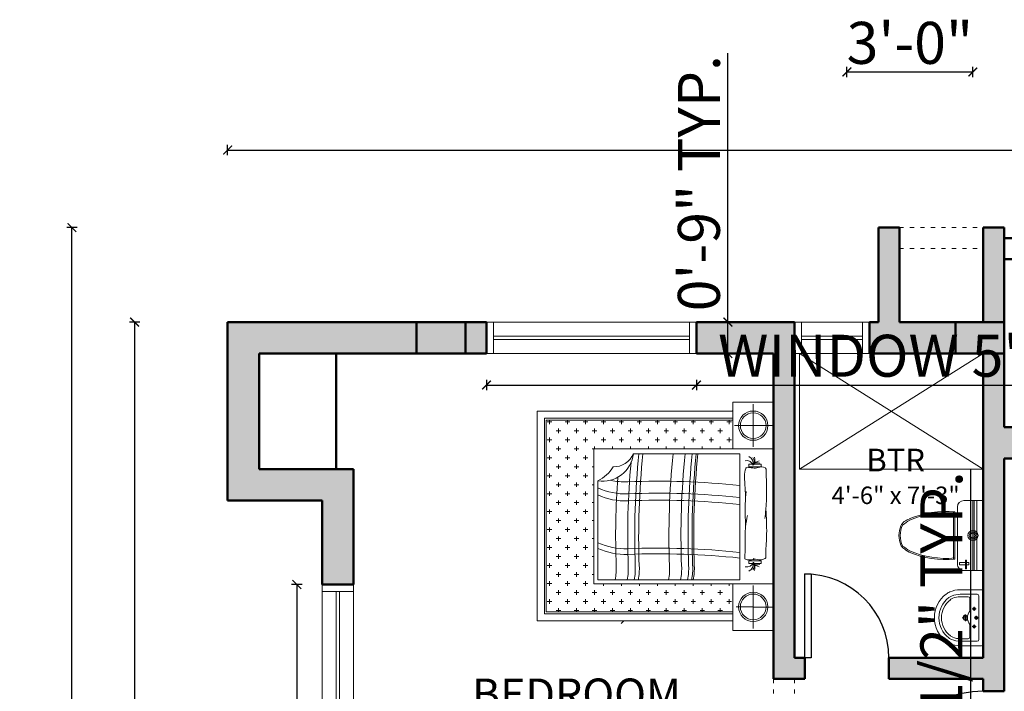
# Model space of a CAD drawing. Units: inches. Extents: x 375 to 1122, y 27 to 1069.
# Tile 77 of 155: x 385 to 667, y 877 to 1069. Entities that reach past the tile are written whole.
import ezdxf

# ---------------------------------------------------------------- set-up
doc = ezdxf.new("R2010")
doc.units = ezdxf.units.IN
doc.linetypes.add('ACAD_ISO03W100', pattern=[30, 12, -18])
for name, color, linetype, lineweight in [('A-ANNO-DIMS', 2, 'Continuous', 18), ('A-AREA-IDEN', 7, 'Continuous', 18), ('A-COLS-PATT', 10, 'Continuous', 13), ('A-FLOR-FIXT', 55, 'Continuous', 18), ('A-WALL-OVHD', 77, 'ACAD_ISO03W100', 18), ('A-WALL-PATT', 252, 'Continuous', 13), ('Columns', 10, 'Continuous', 50), ('Doors', 150, 'Continuous', 25), ('Furniture', 30, 'Continuous', 18), ('Shower Areas', 53, 'Continuous', 18), ('Walls', 250, 'Continuous', 50), ('Windows', 122, 'Continuous', 18)]:
    doc.layers.add(name, color=color, linetype=linetype, lineweight=lineweight)
doc.styles.get("Standard").update_dxf_attribs({"font": 'arial.ttf'})
doc.dimstyles.new('ISO-25', dxfattribs={"dimtxt": 12, "dimasz": 2.5, "dimexe": 1.5, "dimexo": 1.5, "dimtad": 1, "dimdec": 1, "dimlunit": 3, "dimtxsty": 'Standard', "dimblk": 'ARCHTICK', "dimcen": 2.5, "dimadec": 0, "dimazin": 0, "dimtfac": 1, "dimtdec": 1, "dimtmove": 0, "dimatfit": 3, "dimfxl": 1.5, "dimfxlon": 1, "dimarcsym": 0})

# ---------------------------------------------------------------- blocks, each defined once
blk = doc.blocks.new('*U7')
for p, q in [((0, 0), (0, -4)), ((24, 0), (24, -4))]:
    blk.add_line(p, q)
blk.add_lwpolyline([(0, 0), (0, 24), (1.75, 24), (1.75, 0)], close=True)
blk.add_arc((0, 0), 24, 0, 90)
blk = doc.blocks.new('*U10')
for p, q in [((-30, 0), (-30, 4)), ((0, 0), (0, 4))]:
    blk.add_line(p, q)
blk.add_lwpolyline([(0, 0), (0, -30), (-1.75, -30), (-1.75, 0)], close=True)
blk.add_arc((0, 0), 30, 180, 270)
blk = doc.blocks.new('A$C52B64FF5')
for p, q in [((0.522, 2.628), (0, 2.628)), ((0, 2.628), (0, 2.178)), ((0.262, 2.403), (0.262, 2.616)), ((0.522, 2.178), (0.522, 2.628)), ((2.022, 2.628), (0.522, 2.628)), ((0.522, 2.628), (0.522, 0.628)), ((2.543, 2.628), (2.022, 2.628)), ((2.022, 0.628), (2.022, 2.628)), ((2.022, 2.628), (2.022, 2.178)), ((2.282, 2.403), (2.282, 2.616)), ((2.543, 2.178), (2.543, 2.628)), ((0.721, 2.493), (0.692, 2.493)), ((0.692, 2.493), (0.692, 2.353)), ((0.721, 2.353), (0.721, 2.493)), ((1.767, 2.353), (1.767, 2.493)), ((1.767, 2.493), (1.796, 2.493)), ((1.796, 2.493), (1.796, 2.353)), ((0.263, 2.403), (0.023, 2.403)), ((0.023, 2.403), (0.5, 2.403)), ((0.263, 2.195), (0.263, 2.403)), ((0.692, 2.353), (0.721, 2.353)), ((1.796, 2.353), (1.767, 2.353)), ((2.52, 2.403), (2.043, 2.403)), ((2.28, 2.213), (2.28, 2.403)), ((2.28, 2.403), (2.52, 2.403)), ((0.575, 1.068), (0.575, 2.254)), ((0.575, 2.254), (1.978, 2.254)), ((1.978, 2.254), (1.978, 0.675)), ((0, 2.178), (0.522, 2.178)), ((0.093, 2.178), (0.101, 2.17)), ((0.101, 0), (0.101, 2.178)), ((0.181, 0.08), (0.181, 2.178)), ((0.201, 0.1), (0.201, 2.178)), ((0.201, 2.136), (0.245, 2.136)), ((0.22, 2.111), (0.22, 2.161)), ((0.395, 2.136), (0.445, 2.136)), ((0.42, 2.111), (0.42, 2.161)), ((2.543, 2.178), (2.022, 2.178)), ((2.022, 2.178), (2.543, 2.178)), ((2.022, 2.136), (2.045, 2.136)), ((2.195, 2.136), (2.245, 2.136)), ((2.22, 2.111), (2.22, 2.161)), ((2.337, 2.178), (2.337, 0.1)), ((2.357, 2.178), (2.357, 0.08)), ((2.437, 2.178), (2.437, 0)), ((0.295, 2.036), (0.345, 2.036)), ((0.32, 2.011), (0.32, 2.061)), ((0.495, 2.036), (0.522, 2.036)), ((0.52, 2.011), (0.52, 2.061)), ((2.095, 2.036), (2.145, 2.036)), ((2.12, 2.011), (2.12, 2.061)), ((2.295, 2.036), (2.337, 2.036)), ((2.32, 2.011), (2.32, 2.061)), ((0.201, 1.936), (0.245, 1.936)), ((0.22, 1.911), (0.22, 1.961)), ((0.395, 1.936), (0.445, 1.936)), ((0.42, 1.911), (0.42, 1.961)), ((2.022, 1.936), (2.045, 1.936)), ((2.195, 1.936), (2.245, 1.936)), ((2.22, 1.911), (2.22, 1.961)), ((0.22, 1.711), (0.22, 1.761)), ((0.295, 1.836), (0.345, 1.836)), ((0.32, 1.811), (0.32, 1.861)), ((0.42, 1.711), (0.42, 1.761)), ((0.495, 1.836), (0.522, 1.836)), ((0.52, 1.811), (0.52, 1.861)), ((2.095, 1.836), (2.145, 1.836)), ((2.12, 1.811), (2.12, 1.861)), ((2.22, 1.711), (2.22, 1.761)), ((2.295, 1.836), (2.337, 1.836)), ((2.32, 1.811), (2.32, 1.861)), ((0.201, 1.736), (0.245, 1.736)), ((0.32, 1.611), (0.32, 1.661)), ((0.395, 1.736), (0.445, 1.736)), ((0.52, 1.611), (0.52, 1.661)), ((2.022, 1.736), (2.045, 1.736)), ((2.12, 1.611), (2.12, 1.661)), ((2.195, 1.736), (2.245, 1.736)), ((2.32, 1.611), (2.32, 1.661)), ((0.201, 1.536), (0.245, 1.536)), ((0.22, 1.511), (0.22, 1.561)), ((0.295, 1.636), (0.345, 1.636)), ((0.395, 1.536), (0.445, 1.536)), ((0.42, 1.511), (0.42, 1.561)), ((0.495, 1.636), (0.522, 1.636)), ((2.022, 1.536), (2.045, 1.536)), ((2.095, 1.636), (2.145, 1.636)), ((2.195, 1.536), (2.245, 1.536)), ((2.22, 1.511), (2.22, 1.561)), ((2.295, 1.636), (2.337, 1.636)), ((0.295, 1.436), (0.345, 1.436)), ((0.32, 1.411), (0.32, 1.461)), ((0.495, 1.436), (0.522, 1.436)), ((0.52, 1.411), (0.52, 1.461)), ((2.095, 1.436), (2.145, 1.436)), ((2.12, 1.411), (2.12, 1.461)), ((2.295, 1.436), (2.337, 1.436)), ((2.32, 1.411), (2.32, 1.461)), ((0.201, 1.336), (0.245, 1.336)), ((0.22, 1.311), (0.22, 1.361)), ((0.395, 1.336), (0.445, 1.336)), ((0.42, 1.311), (0.42, 1.361)), ((2.022, 1.336), (2.045, 1.336)), ((2.195, 1.336), (2.245, 1.336)), ((2.22, 1.311), (2.22, 1.361)), ((0.295, 1.236), (0.345, 1.236)), ((0.32, 1.211), (0.32, 1.261)), ((0.495, 1.236), (0.522, 1.236)), ((0.52, 1.211), (0.52, 1.261)), ((2.095, 1.236), (2.145, 1.236)), ((2.12, 1.211), (2.12, 1.261)), ((2.295, 1.236), (2.337, 1.236)), ((2.32, 1.211), (2.32, 1.261)), ((0.201, 1.136), (0.245, 1.136)), ((0.22, 1.111), (0.22, 1.161)), ((0.395, 1.136), (0.445, 1.136)), ((0.42, 1.111), (0.42, 1.161)), ((2.022, 1.136), (2.045, 1.136)), ((2.195, 1.136), (2.245, 1.136)), ((2.22, 1.111), (2.22, 1.161)), ((0.295, 1.036), (0.345, 1.036)), ((0.32, 1.011), (0.32, 1.061)), ((0.495, 1.036), (0.522, 1.036)), ((0.52, 1.011), (0.52, 1.061)), ((2.095, 1.036), (2.145, 1.036)), ((2.12, 1.011), (2.12, 1.061)), ((2.295, 1.036), (2.337, 1.036)), ((2.32, 1.011), (2.32, 1.061)), ((0.201, 0.936), (0.245, 0.936)), ((0.22, 0.911), (0.22, 0.961)), ((0.395, 0.936), (0.445, 0.936)), ((0.42, 0.911), (0.42, 0.961)), ((2.022, 0.936), (2.045, 0.936)), ((2.195, 0.936), (2.245, 0.936)), ((2.22, 0.911), (2.22, 0.961)), ((2.437, 0.962), (2.464, 0.935)), ((0.295, 0.836), (0.345, 0.836)), ((0.32, 0.811), (0.32, 0.861)), ((0.495, 0.836), (0.522, 0.836)), ((0.52, 0.811), (0.52, 0.861)), ((2.095, 0.836), (2.145, 0.836)), ((2.12, 0.811), (2.12, 0.861)), ((2.295, 0.836), (2.337, 0.836)), ((2.32, 0.811), (2.32, 0.861)), ((0.201, 0.736), (0.245, 0.736)), ((0.22, 0.711), (0.22, 0.761)), ((0.32, 0.611), (0.32, 0.661)), ((0.395, 0.736), (0.445, 0.736)), ((0.42, 0.711), (0.42, 0.761)), ((0.52, 0.611), (0.52, 0.661)), ((1.978, 0.675), (0.876, 0.675)), ((2.022, 0.736), (2.045, 0.736)), ((2.12, 0.611), (2.12, 0.661)), ((2.195, 0.736), (2.245, 0.736)), ((2.22, 0.711), (2.22, 0.761)), ((2.32, 0.611), (2.32, 0.661)), ((0.22, 0.511), (0.22, 0.561)), ((0.295, 0.636), (0.345, 0.636)), ((0.42, 0.511), (0.42, 0.561)), ((0.495, 0.636), (0.522, 0.636)), ((0.522, 0.628), (2.022, 0.628)), ((0.62, 0.511), (0.62, 0.561)), ((0.72, 0.611), (0.72, 0.628)), ((0.82, 0.511), (0.82, 0.561)), ((0.92, 0.611), (0.92, 0.628)), ((1.02, 0.511), (1.02, 0.561)), ((1.12, 0.611), (1.12, 0.628)), ((1.22, 0.511), (1.22, 0.561)), ((1.32, 0.611), (1.32, 0.628)), ((1.42, 0.511), (1.42, 0.561)), ((1.52, 0.611), (1.52, 0.628)), ((1.62, 0.511), (1.62, 0.561)), ((1.72, 0.611), (1.72, 0.628)), ((1.82, 0.511), (1.82, 0.561)), ((1.92, 0.611), (1.92, 0.628)), ((2.02, 0.511), (2.02, 0.561)), ((2.095, 0.636), (2.145, 0.636)), ((2.22, 0.511), (2.22, 0.561)), ((2.295, 0.636), (2.337, 0.636)), ((0.201, 0.536), (0.245, 0.536)), ((0.32, 0.411), (0.32, 0.461)), ((0.395, 0.536), (0.445, 0.536)), ((0.52, 0.411), (0.52, 0.461)), ((0.595, 0.536), (0.645, 0.536)), ((0.72, 0.411), (0.72, 0.461)), ((0.795, 0.536), (0.845, 0.536)), ((0.92, 0.411), (0.92, 0.461)), ((0.995, 0.536), (1.045, 0.536)), ((1.12, 0.411), (1.12, 0.461)), ((1.195, 0.536), (1.245, 0.536)), ((1.32, 0.411), (1.32, 0.461)), ((1.395, 0.536), (1.445, 0.536)), ((1.52, 0.411), (1.52, 0.461)), ((1.595, 0.536), (1.645, 0.536)), ((1.72, 0.411), (1.72, 0.461)), ((1.795, 0.536), (1.845, 0.536)), ((1.92, 0.411), (1.92, 0.461)), ((1.995, 0.536), (2.045, 0.536)), ((2.12, 0.411), (2.12, 0.461)), ((2.195, 0.536), (2.245, 0.536)), ((2.32, 0.411), (2.32, 0.461)), ((0.201, 0.336), (0.245, 0.336)), ((0.22, 0.311), (0.22, 0.361)), ((0.295, 0.436), (0.345, 0.436)), ((0.395, 0.336), (0.445, 0.336)), ((0.42, 0.311), (0.42, 0.361)), ((0.495, 0.436), (0.545, 0.436)), ((0.595, 0.336), (0.645, 0.336)), ((0.62, 0.311), (0.62, 0.361)), ((0.695, 0.436), (0.745, 0.436)), ((0.795, 0.336), (0.845, 0.336)), ((0.82, 0.311), (0.82, 0.361)), ((0.895, 0.436), (0.945, 0.436)), ((0.995, 0.336), (1.045, 0.336)), ((1.02, 0.311), (1.02, 0.361)), ((1.095, 0.436), (1.145, 0.436)), ((1.195, 0.336), (1.245, 0.336)), ((1.22, 0.311), (1.22, 0.361)), ((1.295, 0.436), (1.345, 0.436)), ((1.395, 0.336), (1.445, 0.336)), ((1.42, 0.311), (1.42, 0.361)), ((1.495, 0.436), (1.545, 0.436)), ((1.595, 0.336), (1.645, 0.336)), ((1.62, 0.311), (1.62, 0.361)), ((1.695, 0.436), (1.745, 0.436)), ((1.795, 0.336), (1.845, 0.336)), ((1.82, 0.311), (1.82, 0.361)), ((1.895, 0.436), (1.945, 0.436)), ((1.995, 0.336), (2.045, 0.336)), ((2.02, 0.311), (2.02, 0.361)), ((2.095, 0.436), (2.145, 0.436)), ((2.195, 0.336), (2.245, 0.336)), ((2.22, 0.311), (2.22, 0.361)), ((2.295, 0.436), (2.337, 0.436)), ((0.295, 0.236), (0.345, 0.236)), ((0.32, 0.211), (0.32, 0.261)), ((0.495, 0.236), (0.545, 0.236)), ((0.52, 0.211), (0.52, 0.261)), ((0.695, 0.236), (0.745, 0.236)), ((0.72, 0.211), (0.72, 0.261)), ((0.895, 0.236), (0.945, 0.236)), ((0.92, 0.211), (0.92, 0.261)), ((1.095, 0.236), (1.145, 0.236)), ((1.12, 0.211), (1.12, 0.261)), ((1.295, 0.236), (1.345, 0.236)), ((1.32, 0.211), (1.32, 0.261)), ((1.495, 0.236), (1.545, 0.236)), ((1.52, 0.211), (1.52, 0.261)), ((1.695, 0.236), (1.745, 0.236)), ((1.72, 0.211), (1.72, 0.261)), ((1.895, 0.236), (1.945, 0.236)), ((1.92, 0.211), (1.92, 0.261)), ((2.095, 0.236), (2.145, 0.236)), ((2.12, 0.211), (2.12, 0.261)), ((2.295, 0.236), (2.337, 0.236)), ((2.32, 0.211), (2.32, 0.261)), ((0.201, 0.136), (0.245, 0.136)), ((0.22, 0.111), (0.22, 0.161)), ((0.395, 0.136), (0.445, 0.136)), ((0.42, 0.111), (0.42, 0.161)), ((0.595, 0.136), (0.645, 0.136)), ((0.62, 0.111), (0.62, 0.161)), ((0.795, 0.136), (0.845, 0.136)), ((0.82, 0.111), (0.82, 0.161)), ((0.995, 0.136), (1.045, 0.136)), ((1.02, 0.111), (1.02, 0.161)), ((1.195, 0.136), (1.245, 0.136)), ((1.22, 0.111), (1.22, 0.161)), ((1.395, 0.136), (1.445, 0.136)), ((1.42, 0.111), (1.42, 0.161)), ((1.595, 0.136), (1.645, 0.136)), ((1.62, 0.111), (1.62, 0.161)), ((1.795, 0.136), (1.845, 0.136)), ((1.82, 0.111), (1.82, 0.161)), ((1.995, 0.136), (2.045, 0.136)), ((2.02, 0.111), (2.02, 0.161)), ((2.195, 0.136), (2.245, 0.136)), ((2.22, 0.111), (2.22, 0.161)), ((2.437, 0), (0.101, 0)), ((2.357, 0.08), (0.181, 0.08)), ((2.337, 0.1), (0.201, 0.1))]:
    blk.add_line(p, q)
for centre, radius in [((0.263, 2.403), 0.163), ((0.263, 2.403), 0.143), ((2.28, 2.403), 0.163), ((2.28, 2.403), 0.143)]:
    blk.add_circle(centre, radius)
for centre, radius, start, end in [((0.644, 2.315), 0.107, 59.2174, 107.2401), ((0.665, 2.321), 0.0913, 67.8398, 120.4859), ((0.752, 2.492), 0.101, 192.774, 239.2386), ((0.757, 2.452), 0.0808, 161.4559, 221.5545), ((1.736, 2.492), 0.101, 300.7614, 347.226), ((1.844, 2.315), 0.107, 72.7599, 120.7826), ((1.823, 2.321), 0.0913, 59.5141, 112.1602), ((1.732, 2.452), 0.0808, 318.4455, 18.5441), ((0.689, 2.306), 0.098, 80.9486, 149.4879), ((0.729, 2.33), 0.0776, 109.2642, 192.2669), ((1.759, 2.33), 0.0776, 347.7331, 73.8836), ((1.799, 2.306), 0.098, 30.5121, 99.0514), ((9.729, 1.341), 8.848, 174.0754, 182.1662), ((9.863, 1.341), 8.848, 174.0754, 182.1662), ((9.941, 1.341), 8.848, 174.0754, 182.1662), ((10.474, 1.341), 8.848, 174.0754, 182.1662), ((10.537, 1.341), 8.848, 174.0754, 182.1662), ((1.488, 10.589), 8.848, 264.0754, 272.1662), ((1.488, 10.57), 8.848, 264.0754, 272.1662), ((1.488, 10.526), 8.848, 264.0754, 272.1662), ((1.488, 10.447), 8.848, 264.0754, 272.1662), ((1.85, 1.028), 0.72, 79.7409, 92.1662), ((1.85, 1.01), 0.72, 79.7409, 92.1662), ((1.85, 0.965), 0.72, 79.7409, 92.1662), ((1.85, 0.887), 0.72, 79.7409, 92.1662), ((1.488, 10.313), 8.848, 264.0754, 272.1662), ((1.85, 0.753), 0.72, 79.7409, 92.1662), ((1.488, 9.976), 8.848, 264.0754, 272.1662), ((1.488, 9.932), 8.848, 264.0754, 272.1662), ((1.85, 0.416), 0.72, 79.7409, 92.1662), ((0.487, 0.852), 0.234, 358.0368, 67.7864), ((0.539, 0.729), 0.342, 350.9267, 83.9565), ((1.488, 9.854), 8.848, 264.7058, 272.1662), ((0.169, 0.979), 0.72, 346.8653, 2.1662), ((0.303, 0.979), 0.72, 334.9836, 2.1662), ((0.381, 0.979), 0.72, 334.9836, 2.1662), ((0.913, 0.979), 0.72, 334.9836, 2.1662), ((0.976, 0.979), 0.72, 334.9836, 2.1662), ((1.85, 0.371), 0.72, 79.7409, 92.1662), ((1.85, 0.293), 0.72, 79.7409, 92.1662), ((1.488, 9.72), 8.848, 265.7785, 272.1662), ((1.85, 0.159), 0.72, 79.7409, 92.1662), ((0.528, 0.51), 0.385, 25.3912, 60.0686)]:
    blk.add_arc(centre, radius, start, end)
for points, knots in [([(0.737, 2.429), (0.734, 2.439), (0.724, 2.472), (0.715, 2.518), (0.741, 2.546), (0.909, 2.551), (1.086, 2.559), (1.264, 2.536), (1.298, 2.532)], [0, 0, 0, 0, 0.0298664, 0.1071619, 0.1152509, 0.1416099, 0.5761797, 0.6768951, 0.6768951, 0.6768951, 0.6768951]), ([(1.195, 2.544), (1.285, 2.549), (1.448, 2.559), (1.628, 2.543), (1.718, 2.544), (1.735, 2.544)], [0, 0, 0, 0, 0.2717358, 0.4891854, 0.5406465, 0.5406465, 0.5406465, 0.5406465]), ([(1.735, 2.544), (1.742, 2.532), (1.759, 2.501), (1.758, 2.462), (1.735, 2.382), (1.745, 2.415), (1.749, 2.426)], [0, 0, 0, 0, 0.0383771, 0.1013156, 0.1484959, 0.1756343, 0.1756343, 0.1756343, 0.1756343]), ([(1.08, 2.318), (1.023, 2.316), (0.91, 2.312), (0.791, 2.299), (0.723, 2.328), (0.731, 2.377), (0.735, 2.409), (0.737, 2.429)], [0, 0, 0, 0, 0.1744349, 0.3406483, 0.347042, 0.3874998, 0.4538558, 0.4538558, 0.4538558, 0.4538558]), ([(1.749, 2.426), (1.753, 2.408), (1.76, 2.375), (1.757, 2.336), (1.744, 2.306), (1.668, 2.315), (1.559, 2.311), (1.403, 2.312), (1.305, 2.33), (1.263, 2.338)], [0, 0, 0, 0, 0.0550284, 0.1011576, 0.1178362, 0.1437253, 0.3009935, 0.4726259, 0.6000038, 0.6000038, 0.6000038, 0.6000038]), ([(1.375, 2.318), (1.295, 2.315), (1.168, 2.311), (1.041, 2.32), (0.995, 2.323)], [0, 0, 0, 0, 0.2401688, 0.38052, 0.38052, 0.38052, 0.38052])]:
    blk.add_open_spline(points, degree=3, knots=knots)
blk = doc.blocks.new('A$C00C51FE0')
at = {"ltscale": 2}
for p, q in [((16.79, 8.49), (3.21, 8.49)), ((1.59, 4.18), (1.59, 6.81)), ((1.59, 6.81), (2.25, 6.81)), ((1.85, 7.41), (18.15, 7.41)), ((2.25, 6.81), (2.25, 4.18)), ((16.79, 8.12), (3.21, 8.12)), ((0, 0), (0, 5.56)), ((20, 2.96), (0, 2.96)), ((0.5, 4.84), (0.5, 5.06)), ((0.5, 5.06), (2.91, 5.06)), ((2.91, 4.84), (0.5, 4.84)), ((2.25, 4.18), (1.59, 4.18)), ((2.91, 5.06), (2.91, 4.84)), ((20, 5.56), (20, 0)), ((20, 2.59), (0, 2.59)), ((20, 1.85), (0, 1.85)), ((20, 0), (0, 0))]:
    blk.add_line(p, q, dxfattribs=at)
for radius in [1.44, 1.07, 0.698]:
    blk.add_circle((10, 2.96), radius, dxfattribs=at)
for centre, radius, start, end in [((22.68, 10.69), 20.34, 142.816, 148.8373), ((22.68, 10.69), 19.97, 141.7352, 148.8373), ((7.96, 21.86), 1.85, 112.9199, 142.816), ((10, 17.03), 6.73, 63.5839, 116.4161), ((10, 17.03), 7.1, 67.0801, 112.9199), ((11.04, 20.15), 3.83, 16.1902, 63.2078), ((-2.68, 10.69), 19.97, 31.1627, 38.2648), ((29.69, 10.65), 26.6, 156.5869, 185.4494), ((29.69, 10.65), 26.23, 156.5869, 185.4494), ((-9.69, 10.65), 26.23, 354.5506, 23.4131), ((-9.69, 10.65), 26.6, 354.5506, 23.4131), ((1.85, 5.56), 1.85, 90, 180), ((18.15, 5.56), 1.85, 0, 90)]:
    blk.add_arc(centre, radius, start, end, dxfattribs=at)
blk = doc.blocks.new('_ArchTick')
at = {"color": 0, "linetype": 'ByBlock', "const_width": 0.15}
blk.add_lwpolyline([(-0.5, -0.5), (0.5, 0.5)], dxfattribs=at)
blk = doc.blocks.new('*D27')
at = {"layer": 'A-ANNO-DIMS', "color": 0, "lineweight": -2, "transparency": 16777216}
for p, q in [((444.51, 1030.21), (444.51, 1033.21)), ((986.01, 1030.21), (986.01, 1033.21)), ((444.51, 1031.71), (986.01, 1031.71))]:
    blk.add_line(p, q, dxfattribs=at)
at = {"layer": 'Defpoints', "color": 0, "transparency": 16777216}
for p in [(986.01, 1031.71), (444.51, 982.53), (986.01, 982.53)]:
    blk.add_point(p, dxfattribs=at)
at = {"layer": 'A-ANNO-DIMS', "color": 0, "lineweight": -2, "transparency": 16777216, "xscale": 2.5, "yscale": 2.5, "zscale": 2.5, "rotation": 180}
blk.add_blockref('_ArchTick', (444.51, 1031.71), dxfattribs=at)
at = {"layer": 'A-ANNO-DIMS', "color": 0, "lineweight": -2, "transparency": 16777216, "xscale": 2.5, "yscale": 2.5, "zscale": 2.5}
blk.add_blockref('_ArchTick', (986.01, 1031.71), dxfattribs=at)
at = {"layer": 'A-ANNO-DIMS', "color": 0, "transparency": 16777216, "insert": (715.26, 1038.46), "char_height": 12, "attachment_point": 5}
blk.add_mtext('45\'-1.5"', dxfattribs=at)
blk = doc.blocks.new('*D28')
at = {"layer": 'A-ANNO-DIMS', "color": 0, "lineweight": -2, "transparency": 16777216}
for p, q in [((419.42, 982.53), (416.42, 982.53)), ((417.92, 982.53), (417.92, 187.53)), ((419.42, 187.53), (416.42, 187.53))]:
    blk.add_line(p, q, dxfattribs=at)
at = {"layer": 'Defpoints', "color": 0, "transparency": 16777216}
for p in [(444.51, 982.53), (417.92, 187.53), (444.51, 187.53)]:
    blk.add_point(p, dxfattribs=at)
at = {"layer": 'A-ANNO-DIMS', "color": 0, "lineweight": -2, "transparency": 16777216, "xscale": 2.5, "yscale": 2.5, "zscale": 2.5}
for p, rotation in [((417.92, 982.53), 90), ((417.92, 187.53), 270)]:
    blk.add_blockref('_ArchTick', p, dxfattribs=dict(at, rotation=rotation))
at = {"layer": 'A-ANNO-DIMS', "color": 0, "transparency": 16777216, "insert": (411.17, 585.03), "char_height": 12, "attachment_point": 5, "rotation": 90}
blk.add_mtext('66\'-3"', dxfattribs=at)
blk = doc.blocks.new('WINDOW-48IN')
for p, q in [((2, 5), (46, 5)), ((2, 4), (46, 4))]:
    blk.add_line(p, q)
blk.add_lwpolyline([(48, 0), (0, 0), (0, 9), (48, 9)], close=True)
for points in [[(2, 0), (2, 9)], [(46, 9), (46, 0)]]:
    blk.add_lwpolyline(points)
blk = doc.blocks.new('WINDOW-21_5IN')
for p, q in [((4, 2), (4, 19.5)), ((5, 2), (5, 19.5))]:
    blk.add_line(p, q)
blk.add_lwpolyline([(0, 0), (9, 0), (9, 21.5), (0, 21.5)], close=True)
for points in [[(9, 19.5), (0, 19.5)], [(0, 2), (9, 2)]]:
    blk.add_lwpolyline(points)
blk = doc.blocks.new('WINDOW-60IN')
for p, q in [((58, 5), (2, 5)), ((58, 4), (2, 4))]:
    blk.add_line(p, q)
blk.add_lwpolyline([(60, 0), (0, 0), (0, 9), (60, 9)], close=True)
for points in [[(2, 0), (2, 9)], [(58, 9), (58, 0)]]:
    blk.add_lwpolyline(points)
blk = doc.blocks.new('LAVATORY-16IN')
for p, q in [((1.27, 7.37), (1.27, 12.19)), ((1.78, 12.7), (14.22, 12.7)), ((4.89, 11.37), (6.03, 11.37)), ((5.46, 10.79), (5.46, 11.94)), ((7.43, 11.94), (8.57, 11.94)), ((8, 11.37), (8, 12.51)), ((9.97, 11.37), (11.11, 11.37)), ((10.54, 10.79), (10.54, 11.94)), ((14.73, 12.19), (14.73, 7.37)), ((2.01, 7.37), (2.01, 9.65)), ((2.51, 10.16), (6.08, 10.16)), ((7.02, 8.89), (8.98, 8.89)), ((8, 7.91), (8, 9.4)), ((9.91, 10.16), (13.49, 10.16)), ((13.99, 9.65), (13.99, 7.37))]:
    blk.add_line(p, q)
blk.add_lwpolyline([(0.51, 13.97), (15.49, 13.97, -0.414214), (16, 13.46), (16, 7.37, -0.104704), (15.37, 4.36, -0.038376), (14.78, 3.36, -0.495903), (1.22, 3.36, -0.038376), (0.63, 4.36, -0.104704), (0, 7.37), (0, 13.46, -0.414214)], format="xyb", close=True)
for points in [[(1.27, 7.37, 0.102694), (1.78, 4.92, 0.037256), (2.25, 4.11, 0.085618)], [(2.01, 7.37, 0.101044), (2.44, 5.24, 0.036381), (2.84, 4.54, 0.084644)], [(13.16, 4.54, 0.036381), (13.56, 5.24, 0.101044), (13.99, 7.37, 0.11083)], [(13.75, 4.11, 0.037256), (14.22, 4.92, 0.102694), (14.73, 7.37, 0.111333)]]:
    blk.add_lwpolyline(points, format="xyb")
for centre, radius in [((5.46, 11.37), 0.381), ((8, 11.94), 0.444), ((10.54, 11.37), 0.381), ((8, 8.89), 0.508)]:
    blk.add_circle(centre, radius)
for centre, radius, start, end in [((1.78, 12.19), 0.508, 90, 180), ((14.22, 12.19), 0.508, 0, 90), ((2.51, 9.65), 0.508, 90, 180), ((7.99, 12.19), 2.79, 226.6581, 313.3419), ((8, 8.89), 0.762, 133.135, 47.0367), ((13.49, 9.65), 0.508, 0, 90), ((8, 8.52), 7.25, 217.471, 322.529), ((8, 8.52), 6.51, 217.6433, 322.3567)]:
    blk.add_arc(centre, radius, start, end)
blk = doc.blocks.new('COLUMN-14X9IN')
blk.add_lwpolyline([(0, 0), (14, 0), (14, 9), (0, 9)], close=True)
blk = doc.blocks.new('SHOWER-PAN-52_5X33IN')
for p, q in [((0, 33), (52.5, 0)), ((52.5, 33), (0, 0))]:
    blk.add_line(p, q)
blk.add_lwpolyline([(0, 0), (52.5, 0), (52.5, 33), (0, 33)], close=True)
blk = doc.blocks.new('*D47')
at = {"layer": 'A-ANNO-DIMS', "color": 0, "lineweight": -2, "transparency": 16777216}
for p, q in [((465.81, 907.53), (462.81, 907.53)), ((464.31, 907.53), (464.31, 859.53)), ((465.81, 859.53), (462.81, 859.53)), ((464.31, 859.53), (464.31, 703.93))]:
    blk.add_line(p, q, dxfattribs=at)
at = {"layer": 'Defpoints', "color": 0, "transparency": 16777216}
for p in [(471.51, 907.53), (464.31, 859.53), (471.51, 859.53)]:
    blk.add_point(p, dxfattribs=at)
at = {"layer": 'A-ANNO-DIMS', "color": 0, "lineweight": -2, "transparency": 16777216, "xscale": 2.5, "yscale": 2.5, "zscale": 2.5}
for p, rotation in [((464.31, 907.53), 90), ((464.31, 859.53), 270)]:
    blk.add_blockref('_ArchTick', p, dxfattribs=dict(at, rotation=rotation))
at = {"layer": 'A-ANNO-DIMS', "color": 0, "transparency": 16777216, "insert": (457.47, 780.48), "char_height": 12, "attachment_point": 5, "rotation": 90}
blk.add_mtext('WINDOW 4\'-0" TYP.', dxfattribs=at)
blk = doc.blocks.new('*D55')
at = {"layer": 'A-ANNO-DIMS', "color": 0, "lineweight": -2, "transparency": 16777216}
for p, q in [((518.51, 966.03), (518.51, 963.03)), ((578.51, 966.03), (578.51, 963.03)), ((518.51, 964.53), (578.51, 964.53)), ((578.51, 964.53), (734.11, 964.53))]:
    blk.add_line(p, q, dxfattribs=at)
at = {"layer": 'Defpoints', "color": 0, "transparency": 16777216}
for p in [(518.51, 973.53), (578.51, 973.53), (578.51, 964.53)]:
    blk.add_point(p, dxfattribs=at)
at = {"layer": 'A-ANNO-DIMS', "color": 0, "lineweight": -2, "transparency": 16777216, "xscale": 2.5, "yscale": 2.5, "zscale": 2.5, "rotation": 180}
blk.add_blockref('_ArchTick', (518.51, 964.53), dxfattribs=at)
at = {"layer": 'A-ANNO-DIMS', "color": 0, "lineweight": -2, "transparency": 16777216, "xscale": 2.5, "yscale": 2.5, "zscale": 2.5}
blk.add_blockref('_ArchTick', (578.51, 964.53), dxfattribs=at)
at = {"layer": 'A-ANNO-DIMS', "color": 0, "transparency": 16777216, "insert": (657.56, 971.36), "char_height": 12, "attachment_point": 5}
blk.add_mtext('WINDOW 5\'-0" TYP.', dxfattribs=at)
blk = doc.blocks.new('*D56')
at = {"layer": 'A-ANNO-DIMS', "color": 0, "lineweight": -2, "transparency": 16777216}
for p, q in [((587.51, 982.53), (587.51, 1059.42)), ((586.01, 982.53), (589.01, 982.53)), ((587.51, 973.53), (587.51, 982.53)), ((586.01, 973.53), (589.01, 973.53))]:
    blk.add_line(p, q, dxfattribs=at)
at = {"layer": 'Defpoints', "color": 0, "transparency": 16777216}
for p in [(578.51, 982.53), (587.51, 982.53), (578.51, 973.53)]:
    blk.add_point(p, dxfattribs=at)
at = {"layer": 'A-ANNO-DIMS', "color": 0, "lineweight": -2, "transparency": 16777216, "xscale": 2.5, "yscale": 2.5, "zscale": 2.5}
for p, rotation in [((587.51, 982.53), 90), ((587.51, 973.53), 270)]:
    blk.add_blockref('_ArchTick', p, dxfattribs=dict(at, rotation=rotation))
at = {"layer": 'A-ANNO-DIMS', "color": 0, "transparency": 16777216, "insert": (580.76, 1022.23), "char_height": 12, "attachment_point": 5, "rotation": 90}
blk.add_mtext('0\'-9" TYP.', dxfattribs=at)
blk = doc.blocks.new('*D58')
at = {"layer": 'A-ANNO-DIMS', "color": 0, "lineweight": -2, "transparency": 16777216}
for p, q in [((656.91, 835.53), (656.91, 940.29)), ((655.41, 835.53), (658.41, 835.53)), ((656.91, 750.84), (656.91, 835.53)), ((655.41, 750.84), (658.41, 750.84))]:
    blk.add_line(p, q, dxfattribs=at)
at = {"layer": 'Defpoints', "color": 0, "transparency": 16777216}
for p in [(638.07, 835.53), (656.91, 835.53), (638.07, 750.84)]:
    blk.add_point(p, dxfattribs=at)
at = {"layer": 'A-ANNO-DIMS', "color": 0, "lineweight": -2, "transparency": 16777216, "xscale": 2.5, "yscale": 2.5, "zscale": 2.5}
for p, rotation in [((656.91, 835.53), 90), ((656.91, 750.84), 270)]:
    blk.add_blockref('_ArchTick', p, dxfattribs=dict(at, rotation=rotation))
at = {"layer": 'A-ANNO-DIMS', "color": 0, "transparency": 16777216, "insert": (650.08, 889.16), "char_height": 12, "attachment_point": 5, "rotation": 90}
blk.add_mtext('7\'-0 1/2" TYP.', dxfattribs=at)
blk = doc.blocks.new('*D82')
at = {"layer": 'A-ANNO-DIMS', "color": 0, "lineweight": -2, "transparency": 16777216}
for p, q in [((401.51, 1009.53), (398.51, 1009.53)), ((400.01, 160.53), (400.01, 1009.53)), ((401.51, 160.53), (398.51, 160.53))]:
    blk.add_line(p, q, dxfattribs=at)
at = {"layer": 'Defpoints', "color": 0, "transparency": 16777216}
for p in [(400.01, 1009.53), (630.53, 1009.53), (630.53, 160.53)]:
    blk.add_point(p, dxfattribs=at)
at = {"layer": 'A-ANNO-DIMS', "color": 0, "lineweight": -2, "transparency": 16777216, "xscale": 2.5, "yscale": 2.5, "zscale": 2.5}
for p, rotation in [((400.01, 1009.53), 90), ((400.01, 160.53), 270)]:
    blk.add_blockref('_ArchTick', p, dxfattribs=dict(at, rotation=rotation))
at = {"layer": 'A-ANNO-DIMS', "color": 0, "transparency": 16777216, "insert": (393.26, 585.03), "char_height": 12, "attachment_point": 5, "rotation": 90}
blk.add_mtext('70\'-9"', dxfattribs=at)
blk = doc.blocks.new('*D92')
at = {"layer": 'A-ANNO-DIMS', "color": 0, "lineweight": -2, "transparency": 16777216}
for p, q in [((621.51, 1052.53), (621.51, 1055.53)), ((657.51, 1052.53), (657.51, 1055.53)), ((621.51, 1054.03), (657.51, 1054.03))]:
    blk.add_line(p, q, dxfattribs=at)
at = {"layer": 'Defpoints', "color": 0, "transparency": 16777216}
for p in [(657.51, 1054.03), (621.51, 460.53), (657.51, 460.53)]:
    blk.add_point(p, dxfattribs=at)
at = {"layer": 'A-ANNO-DIMS', "color": 0, "lineweight": -2, "transparency": 16777216, "xscale": 2.5, "yscale": 2.5, "zscale": 2.5, "rotation": 180}
blk.add_blockref('_ArchTick', (621.51, 1054.03), dxfattribs=at)
at = {"layer": 'A-ANNO-DIMS', "color": 0, "lineweight": -2, "transparency": 16777216, "xscale": 2.5, "yscale": 2.5, "zscale": 2.5}
blk.add_blockref('_ArchTick', (657.51, 1054.03), dxfattribs=at)
at = {"layer": 'A-ANNO-DIMS', "color": 0, "transparency": 16777216, "insert": (639.51, 1060.78), "char_height": 12, "attachment_point": 5}
blk.add_mtext('3\'-0"', dxfattribs=at)

msp = doc.modelspace()

# ---------------------------------------------------------------- hatches: boundary and pattern name
at = {"layer": 'A-COLS-PATT'}
h = msp.add_hatch(color=256, dxfattribs=at)
h.dxf.hatch_style = 1
h.paths.add_polyline_path([(512.51, 982.53), (498.51, 982.53), (498.51, 973.53), (512.51, 973.53)])
h.paths.add_polyline_path([(666.51, 982.53), (652.51, 982.53), (652.51, 973.53), (666.51, 973.53)])
h.paths.add_polyline_path([(802.01, 982.53), (788.01, 982.53), (788.01, 973.53), (802.01, 973.53)])
h.paths.add_polyline_path([(932.01, 982.53), (918.01, 982.53), (918.01, 973.53), (932.01, 973.53)])
h.paths.add_polyline_path([(507.51, 841.53), (498.51, 841.53), (498.51, 827.53), (507.51, 827.53)])
h.paths.add_polyline_path([(666.51, 844.53), (652.51, 844.53), (652.51, 835.53), (666.51, 835.53)])
h.paths.add_polyline_path([(802.01, 814.53), (788.01, 814.53), (788.01, 805.53), (802.01, 805.53)])
h.paths.add_polyline_path([(932.01, 814.53), (918.01, 814.53), (918.01, 805.53), (932.01, 805.53)])
h.paths.add_polyline_path([(507.51, 719.53), (498.51, 719.53), (498.51, 705.53), (507.51, 705.53)])
h.paths.add_polyline_path([(731.01, 676.53), (722.01, 676.53), (722.01, 662.53), (731.01, 662.53)])
h.paths.add_polyline_path([(802.01, 676.53), (788.01, 676.53), (788.01, 667.53), (802.01, 667.53)])
h.paths.add_polyline_path([(932.01, 676.53), (918.01, 676.53), (918.01, 667.53), (932.01, 667.53)])
h.paths.add_polyline_path([(932.01, 583.53), (918.01, 583.53), (918.01, 574.53), (932.01, 574.53)])
h.paths.add_polyline_path([(868.01, 583.53), (854.01, 583.53), (854.01, 574.53), (868.01, 574.53)])
h.paths.add_polyline_path([(868.01, 502.53), (854.01, 502.53), (854.01, 493.53), (868.01, 493.53)])
h.paths.add_polyline_path([(932.01, 502.53), (918.01, 502.53), (918.01, 493.53), (932.01, 493.53)])
h.paths.add_polyline_path([(672.51, 592.03), (663.51, 592.03), (663.51, 578.03), (672.51, 578.03)])
h.paths.add_polyline_path([(512.51, 589.53), (498.51, 589.53), (498.51, 580.53), (512.51, 580.53)])
h.paths.add_polyline_path([(507.51, 464.53), (498.51, 464.53), (498.51, 450.53), (507.51, 450.53)])
h.paths.add_polyline_path([(731.01, 507.53), (722.01, 507.53), (722.01, 493.53), (731.01, 493.53)])
h.paths.add_polyline_path([(802.01, 502.53), (788.01, 502.53), (788.01, 493.53), (802.01, 493.53)])
h.paths.add_polyline_path([(507.51, 342.53), (498.51, 342.53), (498.51, 328.53), (507.51, 328.53)])
h.paths.add_polyline_path([(512.51, 196.53), (498.51, 196.53), (498.51, 187.53), (512.51, 187.53)])
h.paths.add_polyline_path([(666.51, 334.53), (652.51, 334.53), (652.51, 325.53), (666.51, 325.53)])
h.paths.add_polyline_path([(666.51, 196.53), (652.51, 196.53), (652.51, 187.53), (666.51, 187.53)])
h.paths.add_polyline_path([(805.01, 196.53), (791.01, 196.53), (791.01, 187.53), (805.01, 187.53)])
h.paths.add_polyline_path([(932.01, 196.53), (918.01, 196.53), (918.01, 187.53), (932.01, 187.53)])
h.paths.add_polyline_path([(932.01, 334.53), (918.01, 334.53), (918.01, 325.53), (932.01, 325.53)])
h.paths.add_polyline_path([(805.01, 334.53), (791.01, 334.53), (791.01, 325.53), (805.01, 325.53)])
at = {"layer": 'A-WALL-PATT'}
h = msp.add_hatch(color=256, dxfattribs=at)
h.dxf.hatch_style = 1
h.paths.add_polyline_path([(962.01, 388.53), (989.01, 388.53), (989.01, 394.53), (962.01, 394.53), (932.01, 394.53), (932.01, 397.53), (923.01, 397.53), (923.01, 394.53), (842.01, 394.53), (842.01, 334.53), (839.51, 334.53), (839.51, 328.53), (854.01, 328.53), (854.01, 334.53), (848.01, 334.53), (848.01, 388.53), (953.01, 388.53), (953.01, 356.08), (962.01, 356.08), (962.01, 358.55), (989.01, 358.55), (989.01, 364.55), (962.01, 364.55)])
h.paths.add_polyline_path([(989.01, 502.53), (932.01, 502.53), (932.01, 583.53), (932.01, 593.53), (923.01, 593.53), (923.01, 583.53), (854.01, 583.53), (854.01, 556.53), (863.01, 556.53), (863.01, 574.53), (923.01, 574.53), (923.01, 502.53), (863.01, 502.53), (863.01, 520.53), (854.01, 520.53), (854.01, 502.53), (773.01, 502.53), (773.01, 493.53), (788.01, 493.53), (788.01, 402.03), (722.01, 402.03), (722.01, 373.53), (728.01, 373.53), (728.01, 396.03), (788.01, 396.03), (788.01, 373.53), (794.01, 373.53), (794.01, 430.53), (814.01, 430.53), (814.01, 436.53), (794.01, 436.53), (794.01, 493.53), (923.01, 493.53), (923.01, 487.53), (932.01, 487.53), (932.01, 493.53), (983.01, 493.53), (983.01, 473.53), (989.01, 473.53)])
h.paths.add_polyline_path([(797.01, 325.53), (805.01, 325.53), (805.01, 328.53), (807.51, 328.53), (807.51, 334.53), (791.01, 334.53), (791.01, 226.53), (770.76, 226.53), (770.76, 217.53), (791.01, 217.53), (791.01, 187.53), (855.01, 187.53), (855.01, 196.53), (797.01, 196.53)])
h.paths.add_polyline_path([(989.01, 238.53), (962.01, 238.53), (962.01, 256.42), (953.01, 256.42), (953.01, 229.53), (980.01, 229.53), (980.01, 196.53), (915.01, 196.53), (915.01, 187.53), (989.01, 187.53)])
h.paths.add_polyline_path([(962.01, 334.53), (884.01, 334.53), (884.01, 328.53), (918.01, 328.53), (918.01, 325.53), (932.01, 325.53), (932.01, 328.53), (953.01, 328.53), (953.01, 304.42), (962.01, 304.42)])
h.paths.add_polyline_path([(606.51, 283.53), (609.51, 283.53), (609.51, 289.53), (600.51, 289.53), (600.51, 196.53), (578.51, 196.53), (578.51, 187.53), (606.51, 187.53), (606.51, 196.53)])
h.paths.add_polyline_path([(666.51, 292.53), (660.51, 292.53), (660.51, 289.53), (633.51, 289.53), (633.51, 283.53), (660.51, 283.53), (660.51, 196.53), (628.01, 196.53), (628.01, 187.53), (630.53, 187.53), (630.53, 160.53), (636.53, 160.53), (636.53, 187.53), (660.51, 187.53), (660.51, 160.53), (666.51, 160.53), (666.51, 217.53), (686.76, 217.53), (686.76, 226.53), (666.51, 226.53)])
h.paths.add_polyline_path([(480.51, 256.42), (471.51, 256.42), (471.51, 238.53), (444.51, 238.53), (444.51, 187.53), (518.51, 187.53), (518.51, 196.53), (453.51, 196.53), (453.51, 229.53), (480.51, 229.53)])
h.paths.add_polyline_path([(480.51, 328.53), (652.51, 328.53), (652.51, 325.53), (660.51, 325.53), (660.51, 322.53), (666.51, 322.53), (666.51, 334.53), (507.51, 334.53), (507.51, 360.53), (498.51, 360.53), (498.51, 334.53), (471.51, 334.53), (471.51, 304.42), (480.51, 304.42)])
h.paths.add_polyline_path([(507.51, 484.53), (498.51, 484.53), (498.51, 444.53), (507.51, 444.53), (507.51, 454.53), (621.51, 454.53), (621.51, 460.53), (507.51, 460.53)])
h.paths.add_polyline_path([(672.51, 604.53), (683.26, 604.53), (683.26, 613.53), (669.51, 613.53), (669.51, 649.53), (663.51, 649.53), (663.51, 589.53), (507.51, 589.53), (507.51, 613.53), (498.51, 613.53), (498.51, 556.53), (507.51, 556.53), (507.51, 580.53), (663.51, 580.53), (663.51, 520.53), (669.51, 520.53), (669.51, 556.53), (683.26, 556.53), (683.26, 565.53), (672.51, 565.53)])
h.paths.add_polyline_path([(731.01, 667.53), (734.01, 667.53), (734.01, 676.53), (728.01, 676.53), (728.01, 715.53), (657.51, 715.53), (657.51, 709.53), (663.51, 709.53), (663.51, 673.53), (669.51, 673.53), (669.51, 709.53), (722.01, 709.53), (722.01, 613.53), (704.76, 613.53), (704.76, 604.53), (722.01, 604.53), (722.01, 565.53), (704.76, 565.53), (704.76, 556.53), (722.01, 556.53), (722.01, 502.53), (722.01, 460.53), (669.51, 460.53), (669.51, 496.53), (663.51, 496.53), (663.51, 460.53), (657.51, 460.53), (657.51, 454.53), (728.01, 454.53), (728.01, 493.53), (734.01, 493.53), (734.01, 502.53), (731.01, 502.53)])
h.paths.add_polyline_path([(986.01, 718.53), (959.01, 718.53), (959.01, 727.53), (950.01, 727.53), (950.01, 709.53), (977.01, 709.53), (977.01, 676.53), (794.01, 676.53), (794.01, 805.53), (802.01, 805.53), (802.01, 808.53), (804.51, 808.53), (804.51, 814.53), (788.01, 814.53), (788.01, 774.03), (728.01, 774.03), (728.01, 796.53), (722.01, 796.53), (722.01, 768.03), (788.01, 768.03), (788.01, 676.53), (773.01, 676.53), (773.01, 667.53), (923.01, 667.53), (923.01, 657.53), (932.01, 657.53), (932.01, 667.53), (986.01, 667.53)])
h.paths.add_polyline_path([(621.51, 715.53), (507.51, 715.53), (507.51, 733.53), (498.51, 733.53), (498.51, 715.53), (498.51, 685.53), (507.51, 685.53), (507.51, 709.53), (621.51, 709.53)])
h.paths.add_polyline_path([(666.51, 847.03), (660.51, 847.03), (660.51, 844.53), (652.51, 844.53), (652.51, 841.53), (480.51, 841.53), (480.51, 859.53), (471.51, 859.53), (471.51, 835.53), (498.51, 835.53), (498.51, 817.53), (507.51, 817.53), (507.51, 835.53), (666.51, 835.53)])
h.paths.add_polyline_path([(480.51, 940.53), (453.51, 940.53), (453.51, 973.53), (518.51, 973.53), (518.51, 982.53), (444.51, 982.53), (444.51, 931.53), (471.51, 931.53), (471.51, 907.53), (480.51, 907.53)])
h.paths.add_polyline_path([(606.51, 982.53), (578.51, 982.53), (578.51, 973.53), (600.51, 973.53), (600.51, 880.53), (609.51, 880.53), (609.51, 886.53), (606.51, 886.53)])
h.paths.add_polyline_path([(666.51, 943.53), (686.76, 943.53), (686.76, 952.53), (666.51, 952.53), (666.51, 1009.53), (660.51, 1009.53), (660.51, 982.53), (636.53, 982.53), (636.53, 1009.53), (630.53, 1009.53), (630.53, 982.53), (628.01, 982.53), (628.01, 973.53), (660.51, 973.53), (660.51, 886.53), (633.51, 886.53), (633.51, 880.53), (660.51, 880.53), (660.51, 877.03), (666.51, 877.03)])
h.paths.add_polyline_path([(986.01, 874.53), (932.01, 874.53), (932.01, 877.53), (923.01, 877.53), (923.01, 874.53), (788.01, 874.53), (788.01, 868.53), (788.01, 844.53), (794.01, 844.53), (794.01, 868.53), (839.01, 868.53), (839.01, 814.53), (836.51, 814.53), (836.51, 808.53), (851.01, 808.53), (851.01, 814.53), (845.01, 814.53), (845.01, 868.53), (986.01, 868.53)])
h.paths.add_polyline_path([(959.01, 838.55), (986.01, 838.55), (986.01, 844.55), (959.01, 844.55), (959.01, 847.03), (950.01, 847.03), (950.01, 814.53), (881.01, 814.53), (881.01, 808.53), (918.01, 808.53), (918.01, 805.53), (932.01, 805.53), (932.01, 808.53), (950.01, 808.53), (950.01, 793.53), (959.01, 793.53)])
h.paths.add_polyline_path([(986.01, 982.53), (899.01, 982.53), (899.01, 973.53), (923.01, 973.53), (923.01, 967.53), (932.01, 967.53), (932.01, 973.53), (980.01, 973.53), (980.01, 953.53), (986.01, 953.53)])
h.paths.add_polyline_path([(851.01, 982.53), (788.01, 982.53), (788.01, 952.53), (770.76, 952.53), (770.76, 943.53), (788.01, 943.53), (788.01, 910.53), (814.01, 910.53), (814.01, 916.53), (794.01, 916.53), (794.01, 973.53), (851.01, 973.53)])

# ---------------------------------------------------------------- linework, layer by layer
at = {"layer": 'A-WALL-OVHD', "ltscale": 0.1}
for p, q in [((636.53, 1009.53), (660.51, 1009.53)), ((636.53, 1003.53), (660.51, 1003.53)), ((600.51, 880.53), (600.51, 841.53)), ((606.51, 880.53), (606.51, 841.53))]:
    msp.add_line(p, q, dxfattribs=at)
at = {"layer": 'Walls'}
for p, q in [((630.53, 982.53), (630.53, 1009.53)), ((630.53, 1009.53), (636.53, 1009.53)), ((636.53, 1009.53), (636.53, 982.53)), ((666.51, 1009.53), (660.51, 1009.53)), ((660.51, 1009.53), (660.51, 982.53)), ((666.51, 952.53), (666.51, 1009.53)), ((797.01, 1006.53), (666.51, 1006.53)), ((791.01, 1000.53), (666.51, 1000.53)), ((444.51, 982.53), (444.51, 931.53)), ((444.51, 982.53), (518.51, 982.53)), ((518.51, 973.53), (518.51, 982.53)), ((578.51, 973.53), (578.51, 982.53)), ((578.51, 982.53), (606.51, 982.53)), ((606.51, 886.53), (606.51, 982.53)), ((628.01, 973.53), (628.01, 982.53)), ((628.01, 982.53), (630.53, 982.53)), ((636.53, 982.53), (660.51, 982.53)), ((453.51, 973.53), (453.51, 940.53)), ((518.51, 973.53), (453.51, 973.53)), ((475.51, 973.53), (475.51, 940.53)), ((600.51, 973.53), (578.51, 973.53)), ((600.51, 880.53), (600.51, 973.53)), ((628.01, 973.53), (660.51, 973.53)), ((660.51, 886.53), (660.51, 973.53)), ((686.76, 952.53), (666.51, 952.53)), ((666.51, 877.03), (666.51, 943.53)), ((686.76, 943.53), (666.51, 943.53)), ((453.51, 940.53), (480.51, 940.53)), ((480.51, 940.53), (480.51, 907.53)), ((444.51, 931.53), (471.51, 931.53)), ((471.51, 931.53), (471.51, 907.53)), ((480.51, 907.53), (471.51, 907.53)), ((606.51, 886.53), (609.51, 886.53)), ((609.51, 886.53), (609.51, 880.53)), ((633.51, 886.53), (633.51, 880.53)), ((633.51, 886.53), (660.51, 886.53)), ((600.51, 880.53), (609.51, 880.53)), ((633.51, 880.53), (660.51, 880.53)), ((660.51, 877.03), (660.51, 880.53)), ((660.51, 877.03), (666.51, 877.03))]:
    msp.add_line(p, q, dxfattribs=at)

# ---------------------------------------------------------------- block references
at = {"layer": 'A-FLOR-FIXT'}
for name, p, rotation in [('A$C00C51FE0', (660.51, 911.53), 89.99999999999999), ('LAVATORY-16IN', (646.54, 906.02), 270)]:
    msp.add_blockref(name, p, dxfattribs=dict(at, rotation=rotation))
at = {"layer": 'Columns', "rotation": 180}
for p in [(512.51, 982.53), (666.51, 982.53)]:
    msp.add_blockref('COLUMN-14X9IN', p, dxfattribs=at)
at = {"layer": 'Doors'}
msp.add_blockref('*U7', (609.51, 886.53), dxfattribs=at)
at = {"layer": 'Doors', "rotation": 270}
msp.add_blockref('*U10', (660.51, 847.03), dxfattribs=at)
at = {"layer": 'Furniture', "xscale": 25.67804170018038, "yscale": 25.67804170018038, "zscale": 25.67804170018038, "rotation": 270}
msp.add_blockref('A$C52B64FF5', (533.03, 959.68), dxfattribs=at)
at = {"layer": 'Shower Areas', "extrusion": (0, 0, -1), "zscale": -1, "rotation": 180}
msp.add_blockref('SHOWER-PAN-52_5X33IN', (-608.01, 973.53), dxfattribs=at)
at = {"layer": 'Windows'}
msp.add_blockref('WINDOW-60IN', (518.51, 973.53), dxfattribs=at)
for name, p, rotation in [('WINDOW-21_5IN', (628.01, 973.53), 90), ('WINDOW-48IN', (471.51, 907.53), 270)]:
    msp.add_blockref(name, p, dxfattribs=dict(at, rotation=rotation))

# ---------------------------------------------------------------- texts
at = {"layer": 'A-AREA-IDEN', "attachment_point": 7}
for s, width, insert, char_height in [('\\pxqc;{\\fArial|b1|i0|c0|p34;BTR\\P\\fArial|b0|i0|c0|p34;\\H0.76923x;4\'-6" x 7\'-3"}', 42.2291, (614.34, 930.51), 6.5), ('\\pxqc;{\\fArial|b1|i0|c0|p34;\\H0.75x;BEDROOM\\H1.33333x;\\P\\fArial|b0|i0|c0|p34;\\H0.5x;10\'-0" x 11\'-0"}', 73.8986, (507.26, 859.65), 12)]:
    msp.add_mtext_dynamic_manual_height_columns(s, width=width, gutter_width=12.5, heights=[0], dxfattribs=dict(at, insert=insert, char_height=char_height))

# ---------------------------------------------------------------- dimensions: what is measured, and where the dimension line sits
at = {"layer": 'A-ANNO-DIMS'}
dim = msp.add_linear_dim(base=(657.51, 1054.03), p1=(621.51, 460.53), p2=(657.51, 460.53), dimstyle='ISO-25', override={"dimdec": 1, "dimlfac": 1, "dimrnd": 0, "dimzin": 1, "dimdsep": 46, "dimlunit": 4, "dimfrac": 2}, dxfattribs=at)
dim.commit()
dim.dimension.update_dxf_attribs({"geometry": '*D92', "text_midpoint": (639.51, 1060.78)})
for base, p1, p2, angle, text, picture, middle in [((587.51, 982.53), (578.51, 973.53), (578.51, 982.53), 90, '<> TYP.', '*D56', (580.76, 1022.23)), ((656.91, 835.53), (638.07, 750.84), (638.07, 835.53), 90, '<> TYP.', '*D58', (650.08, 889.16)), ((464.31, 859.53), (471.51, 907.53), (471.51, 859.53), 270, 'WINDOW <> TYP.', '*D47', (457.47, 780.48))]:
    dim = msp.add_linear_dim(base=base, p1=p1, p2=p2, angle=angle, text=text, dimstyle='ISO-25', override={"dimdec": 1, "dimlfac": 1, "dimrnd": 0, "dimzin": 1, "dimdsep": 46, "dimlunit": 4, "dimfrac": 2}, dxfattribs=at)
    dim.commit()
    dim.dimension.update_dxf_attribs({"geometry": picture, "text_midpoint": middle})
dim = msp.add_linear_dim(base=(986.01, 1031.71), p1=(444.51, 982.53), p2=(986.01, 982.53), dimstyle='ISO-25', override={"dimclrd": 0, "dimclre": 0, "dimclrt": 0}, dxfattribs=at)
dim.commit()
dim.dimension.update_dxf_attribs({"geometry": '*D27', "text_midpoint": (715.26, 1031.71), "dimtype": 160})
for base, p1, p2, override, picture, middle in [((400.01, 1009.53), (630.53, 160.53), (630.53, 1009.53), {"dimdec": 1, "dimlfac": 1, "dimrnd": 0, "dimzin": 1, "dimdsep": 46, "dimlunit": 4, "dimfrac": 2}, '*D82', (393.26, 585.03)), ((417.92, 187.53), (444.51, 982.53), (444.51, 187.53), {"dimclrd": 0, "dimclre": 0, "dimclrt": 0}, '*D28', (411.17, 585.03))]:
    dim = msp.add_linear_dim(base=base, p1=p1, p2=p2, angle=90, dimstyle='ISO-25', override=override, dxfattribs=at)
    dim.commit()
    dim.dimension.update_dxf_attribs({"geometry": picture, "text_midpoint": middle})
dim = msp.add_linear_dim(base=(578.51, 964.53), p1=(518.51, 973.53), p2=(578.51, 973.53), text='WINDOW <> TYP.', dimstyle='ISO-25', override={"dimdec": 1, "dimlfac": 1, "dimrnd": 0, "dimzin": 1, "dimdsep": 46, "dimlunit": 4, "dimfrac": 2}, dxfattribs=at)
dim.commit()
dim.dimension.update_dxf_attribs({"geometry": '*D55', "text_midpoint": (657.56, 971.36)})

doc.saveas('drawing.dxf')
